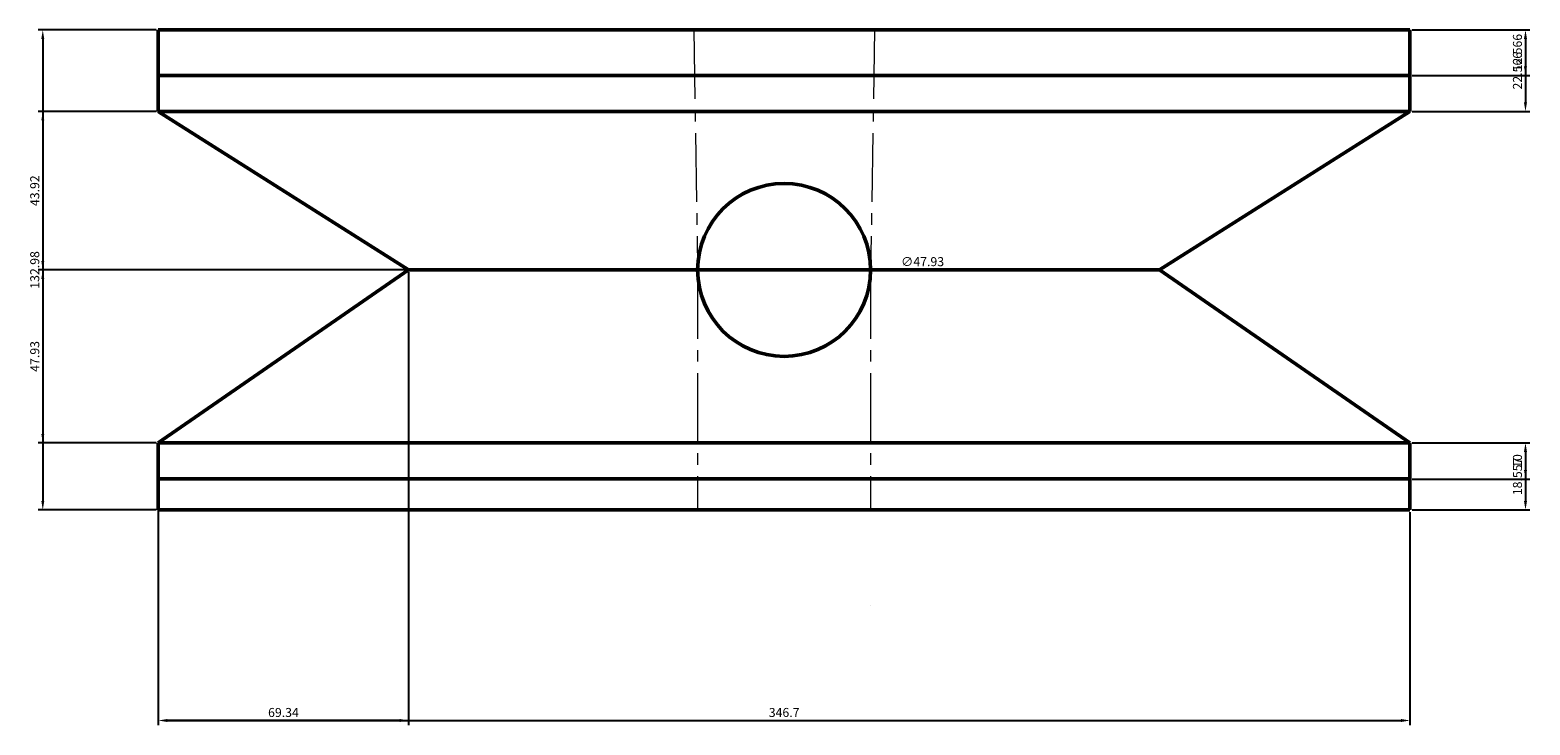
# Model space of a CAD drawing. Units: millimetres. Extents: x 921 to 2648, y 1390 to 2315.
# Tile 7 of 10: x 1771 to 2187, y 1657 to 1849. Entities that reach past the tile are written whole.
import ezdxf

# ---------------------------------------------------------------- set-up
doc = ezdxf.new("R2010")
doc.units = ezdxf.units.MM
doc.linetypes.add('CENTER2', pattern=[28.575, 19.05, -3.175, 3.175, -3.175])
for name, color, linetype, lineweight in [('M-CNTR', 1, 'CENTER2', 18), ('M-DIMS', 2, 'Continuous', 25), ('M-OUTL', 7, 'Continuous', 50)]:
    doc.layers.add(name, color=color, linetype=linetype, lineweight=lineweight)
doc.styles.get("Standard").update_dxf_attribs({"font": 'arial.ttf'})
doc.dimstyles.new('ISO-25', dxfattribs={"dimtxt": 2.5, "dimasz": 2.5, "dimexe": 1.25, "dimexo": 0.625, "dimtad": 1, "dimtxsty": 'Standard', "dimcen": 2.5, "dimadec": 0, "dimazin": 0, "dimtfac": 1, "dimtmove": 0, "dimatfit": 3, "dimfxl": 1, "dimarcsym": 0})

# ---------------------------------------------------------------- blocks, each defined once
blk = doc.blocks.new('*D34')
at = {"layer": 'Defpoints', "color": 0, "transparency": 16777216}
for p in [(1806.98, 1849.47), (1774.98, 1716.49), (1806.98, 1716.49)]:
    blk.add_point(p, dxfattribs=at)
at = {"layer": 'M-DIMS', "color": 0, "lineweight": -2, "transparency": 16777216}
for p, q in [((1806.36, 1849.47), (1773.73, 1849.47)), ((1774.98, 1846.97), (1774.98, 1718.99)), ((1806.36, 1716.49), (1773.73, 1716.49))]:
    blk.add_line(p, q, dxfattribs=at)
at = {"layer": 'M-DIMS', "color": 0, "transparency": 16777216}
for points in [[(1774.57, 1846.97), (1775.4, 1846.97), (1774.98, 1849.47)], [(1774.57, 1718.99), (1775.4, 1718.99), (1774.98, 1716.49)]]:
    blk.add_solid(points, dxfattribs=at)
at = {"layer": 'M-DIMS', "color": 0, "transparency": 16777216, "insert": (1773.08, 1782.98), "char_height": 2.5, "attachment_point": 5, "rotation": 90}
blk.add_mtext('132.98', dxfattribs=at)
blk = doc.blocks.new('*D83')
at = {"layer": 'Defpoints', "color": 0, "transparency": 16777216}
for p in [(1806.98, 1716.49), (2153.69, 1716.49), (2153.69, 1658.13)]:
    blk.add_point(p, dxfattribs=at)
at = {"layer": 'M-DIMS', "color": 0, "lineweight": -2, "transparency": 16777216}
for p, q in [((1806.98, 1715.87), (1806.98, 1656.88)), ((2153.69, 1715.87), (2153.69, 1656.88)), ((1809.48, 1658.13), (2151.19, 1658.13))]:
    blk.add_line(p, q, dxfattribs=at)
at = {"layer": 'M-DIMS', "color": 0, "transparency": 16777216}
for points in [[(1809.48, 1658.55), (1809.48, 1657.72), (1806.98, 1658.13)], [(2151.19, 1658.55), (2151.19, 1657.72), (2153.69, 1658.13)]]:
    blk.add_solid(points, dxfattribs=at)
at = {"layer": 'M-DIMS', "color": 0, "transparency": 16777216, "insert": (1980.34, 1660.03), "char_height": 2.5, "attachment_point": 5}
blk.add_mtext('346.7', dxfattribs=at)
blk = doc.blocks.new('*D84')
at = {"layer": 'Defpoints', "color": 0, "transparency": 16777216}
for p in [(2153.69, 1849.47), (2153.69, 1836.9), (2185.69, 1836.9)]:
    blk.add_point(p, dxfattribs=at)
at = {"layer": 'M-DIMS', "color": 0, "lineweight": -2, "transparency": 16777216}
for p, q in [((2154.32, 1849.47), (2186.94, 1849.47)), ((2185.69, 1846.97), (2185.69, 1839.4)), ((2154.32, 1836.9), (2186.94, 1836.9))]:
    blk.add_line(p, q, dxfattribs=at)
at = {"layer": 'M-DIMS', "color": 0, "transparency": 16777216}
for points in [[(2185.27, 1846.97), (2186.11, 1846.97), (2185.69, 1849.47)], [(2185.27, 1839.4), (2186.11, 1839.4), (2185.69, 1836.9)]]:
    blk.add_solid(points, dxfattribs=at)
at = {"layer": 'M-DIMS', "color": 0, "transparency": 16777216, "insert": (2183.79, 1843.19), "char_height": 2.5, "attachment_point": 5, "rotation": 90}
blk.add_mtext('12.566', dxfattribs=at)
blk = doc.blocks.new('*D85')
at = {"layer": 'Defpoints', "color": 0, "transparency": 16777216}
for p in [(2153.69, 1849.47), (2153.69, 1826.9), (2185.69, 1826.9)]:
    blk.add_point(p, dxfattribs=at)
at = {"layer": 'M-DIMS', "color": 0, "lineweight": -2, "transparency": 16777216}
for p, q in [((2154.32, 1849.47), (2186.94, 1849.47)), ((2185.69, 1846.97), (2185.69, 1829.4)), ((2154.32, 1826.9), (2186.94, 1826.9))]:
    blk.add_line(p, q, dxfattribs=at)
at = {"layer": 'M-DIMS', "color": 0, "transparency": 16777216}
for points in [[(2185.27, 1846.97), (2186.11, 1846.97), (2185.69, 1849.47)], [(2185.27, 1829.4), (2186.11, 1829.4), (2185.69, 1826.9)]]:
    blk.add_solid(points, dxfattribs=at)
at = {"layer": 'M-DIMS', "color": 0, "transparency": 16777216, "insert": (2183.79, 1838.19), "char_height": 2.5, "attachment_point": 5, "rotation": 90}
blk.add_mtext('22.566', dxfattribs=at)
blk = doc.blocks.new('*D86')
at = {"layer": 'Defpoints', "color": 0, "transparency": 16777216}
for p in [(2153.69, 1735.05), (2153.69, 1725.05), (2185.69, 1725.05)]:
    blk.add_point(p, dxfattribs=at)
at = {"layer": 'M-DIMS', "color": 0, "lineweight": -2, "transparency": 16777216}
for p, q in [((2154.32, 1735.05), (2186.94, 1735.05)), ((2185.69, 1732.55), (2185.69, 1727.55)), ((2154.32, 1725.05), (2186.94, 1725.05))]:
    blk.add_line(p, q, dxfattribs=at)
at = {"layer": 'M-DIMS', "color": 0, "transparency": 16777216}
for points in [[(2185.27, 1732.55), (2186.11, 1732.55), (2185.69, 1735.05)], [(2185.27, 1727.55), (2186.11, 1727.55), (2185.69, 1725.05)]]:
    blk.add_solid(points, dxfattribs=at)
at = {"layer": 'M-DIMS', "color": 0, "transparency": 16777216, "insert": (2183.79, 1730.05), "char_height": 2.5, "attachment_point": 5, "rotation": 90}
blk.add_mtext('10', dxfattribs=at)
blk = doc.blocks.new('*D87')
at = {"layer": 'Defpoints', "color": 0, "transparency": 16777216}
for p in [(2153.69, 1735.05), (2153.69, 1716.49), (2185.69, 1716.49)]:
    blk.add_point(p, dxfattribs=at)
at = {"layer": 'M-DIMS', "color": 0, "lineweight": -2, "transparency": 16777216}
for p, q in [((2154.32, 1735.05), (2186.94, 1735.05)), ((2185.69, 1732.55), (2185.69, 1718.99)), ((2154.32, 1716.49), (2186.94, 1716.49))]:
    blk.add_line(p, q, dxfattribs=at)
at = {"layer": 'M-DIMS', "color": 0, "transparency": 16777216}
for points in [[(2185.27, 1732.55), (2186.11, 1732.55), (2185.69, 1735.05)], [(2185.27, 1718.99), (2186.11, 1718.99), (2185.69, 1716.49)]]:
    blk.add_solid(points, dxfattribs=at)
at = {"layer": 'M-DIMS', "color": 0, "transparency": 16777216, "insert": (2183.79, 1725.77), "char_height": 2.5, "attachment_point": 5, "rotation": 90}
blk.add_mtext('18.557', dxfattribs=at)
blk = doc.blocks.new('*D88')
at = {"layer": 'Defpoints', "color": 0, "transparency": 16777216}
for p in [(1806.98, 1826.9), (1774.98, 1782.98), (1876.32, 1782.98)]:
    blk.add_point(p, dxfattribs=at)
at = {"layer": 'M-DIMS', "color": 0, "lineweight": -2, "transparency": 16777216}
for p, q in [((1806.36, 1826.9), (1773.73, 1826.9)), ((1774.98, 1824.4), (1774.98, 1785.48)), ((1875.7, 1782.98), (1773.73, 1782.98))]:
    blk.add_line(p, q, dxfattribs=at)
at = {"layer": 'M-DIMS', "color": 0, "transparency": 16777216}
for points in [[(1774.57, 1824.4), (1775.4, 1824.4), (1774.98, 1826.9)], [(1774.57, 1785.48), (1775.4, 1785.48), (1774.98, 1782.98)]]:
    blk.add_solid(points, dxfattribs=at)
at = {"layer": 'M-DIMS', "color": 0, "transparency": 16777216, "insert": (1773.08, 1804.94), "char_height": 2.5, "attachment_point": 5, "rotation": 90}
blk.add_mtext('43.92', dxfattribs=at)
blk = doc.blocks.new('*D89')
at = {"layer": 'Defpoints', "color": 0, "transparency": 16777216}
for p in [(1876.32, 1782.98), (1774.98, 1735.05), (1806.98, 1735.05)]:
    blk.add_point(p, dxfattribs=at)
at = {"layer": 'M-DIMS', "color": 0, "lineweight": -2, "transparency": 16777216}
for p, q in [((1875.7, 1782.98), (1773.73, 1782.98)), ((1774.98, 1780.48), (1774.98, 1737.55)), ((1806.36, 1735.05), (1773.73, 1735.05))]:
    blk.add_line(p, q, dxfattribs=at)
at = {"layer": 'M-DIMS', "color": 0, "transparency": 16777216}
for points in [[(1774.57, 1780.48), (1775.4, 1780.48), (1774.98, 1782.98)], [(1774.57, 1737.55), (1775.4, 1737.55), (1774.98, 1735.05)]]:
    blk.add_solid(points, dxfattribs=at)
at = {"layer": 'M-DIMS', "color": 0, "transparency": 16777216, "insert": (1773.08, 1759.02), "char_height": 2.5, "attachment_point": 5, "rotation": 90}
blk.add_mtext('47.93', dxfattribs=at)
blk = doc.blocks.new('*D90')
at = {"layer": 'Defpoints', "color": 0, "transparency": 16777216}
for p in [(1876.32, 1782.98), (1806.98, 1735.05), (1806.98, 1658.13)]:
    blk.add_point(p, dxfattribs=at)
at = {"layer": 'M-DIMS', "color": 0, "lineweight": -2, "transparency": 16777216}
for p, q in [((1876.32, 1782.36), (1876.32, 1656.88)), ((1806.98, 1734.43), (1806.98, 1656.88)), ((1873.82, 1658.13), (1809.48, 1658.13))]:
    blk.add_line(p, q, dxfattribs=at)
at = {"layer": 'M-DIMS', "color": 0, "transparency": 16777216}
for points in [[(1809.48, 1658.55), (1809.48, 1657.72), (1806.98, 1658.13)], [(1873.82, 1658.55), (1873.82, 1657.72), (1876.32, 1658.13)]]:
    blk.add_solid(points, dxfattribs=at)
at = {"layer": 'M-DIMS', "color": 0, "transparency": 16777216, "insert": (1841.65, 1660.03), "char_height": 2.5, "attachment_point": 5}
blk.add_mtext('69.34', dxfattribs=at)
blk = doc.blocks.new('*D118')
at = {"layer": 'Defpoints', "color": 0, "transparency": 16777216}
for p in [(1956.37, 1782.98), (2004.3, 1782.98)]:
    blk.add_point(p, dxfattribs=at)
at = {"layer": 'M-DIMS', "color": 0, "lineweight": -2, "transparency": 16777216}
for p, q in [((1953.87, 1782.98), (1951.37, 1782.98)), ((1956.37, 1782.98), (2004.3, 1782.98)), ((2024.89, 1782.98), (2006.8, 1782.98))]:
    blk.add_line(p, q, dxfattribs=at)
at = {"layer": 'M-DIMS', "color": 0, "transparency": 16777216}
for points in [[(1953.87, 1783.4), (1953.87, 1782.57), (1956.37, 1782.98)], [(2006.8, 1783.4), (2006.8, 1782.57), (2004.3, 1782.98)]]:
    blk.add_solid(points, dxfattribs=at)
at = {"layer": 'M-DIMS', "color": 0, "transparency": 16777216, "insert": (2018.68, 1784.95), "char_height": 2.5, "attachment_point": 5, "rotation": 0.0007}
blk.add_mtext('∅47.93', dxfattribs=at)

msp = doc.modelspace()

# ---------------------------------------------------------------- linework, layer by layer
at = {"layer": 'M-CNTR'}
for p, q in [((1955.2929, 1849.4706), (1956.3715, 1782.9827)), ((2005.3813, 1849.4706), (2004.3027, 1782.9827)), ((1956.3715, 1782.9827), (1956.3715, 1716.4948)), ((2004.3027, 1782.9827), (2004.3027, 1716.4948)), ((2004.3027, 1690.1325), (2004.3027, 1690.1325))]:
    msp.add_line(p, q, dxfattribs=at)
at = {"layer": 'M-OUTL'}
for p, q in [((1806.9834, 1849.4706), (2153.6909, 1849.4706)), ((1806.9834, 1849.4706), (1806.9834, 1826.9048)), ((2153.6909, 1849.4706), (2153.6909, 1826.9048)), ((1806.9834, 1836.9048), (2153.6909, 1836.9048)), ((2153.6909, 1826.9048), (1806.9834, 1826.9048)), ((1806.9834, 1826.9048), (1876.3249, 1782.9827)), ((2084.3494, 1782.9827), (2153.6909, 1826.9048)), ((1876.3249, 1782.9827), (1806.9834, 1735.0515)), ((1876.3249, 1782.9827), (2084.3494, 1782.9827)), ((2084.3494, 1782.9827), (2153.6909, 1735.0515)), ((2153.6909, 1735.0515), (1806.9834, 1735.0515)), ((1806.9834, 1735.0515), (1806.9834, 1716.4948)), ((2153.6909, 1735.0515), (2153.6909, 1716.4948)), ((1806.9834, 1725.0515), (2153.6909, 1725.0515)), ((2153.6909, 1716.4948), (1806.9834, 1716.4948))]:
    msp.add_line(p, q, dxfattribs=at)
msp.add_circle((1980.3371, 1782.9827), 23.9656, dxfattribs=at)

# ---------------------------------------------------------------- dimensions: what is measured, and where the dimension line sits
at = {"layer": 'M-DIMS'}
for base, p1, p2, override, picture, middle in [((1774.9834, 1716.4948), (1806.9834, 1849.4706), (1806.9834, 1716.4948), {"dimdec": 2, "dimlfac": 1, "dimrnd": 0, "dimzin": 0, "dimdsep": 46, "dimlunit": 2}, '*D34', (1773.0811, 1782.9827)), ((2185.6909, 1836.9048), (2153.6909, 1849.4706), (2153.6909, 1836.9048), {"dimdec": 3, "dimlfac": 1, "dimrnd": 0, "dimzin": 0, "dimdsep": 46, "dimlunit": 2}, '*D84', (2183.7894, 1843.1877)), ((2185.6909, 1826.9048), (2153.6909, 1849.4706), (2153.6909, 1826.9048), {"dimdec": 3, "dimlfac": 1, "dimrnd": 0, "dimzin": 0, "dimdsep": 46, "dimlunit": 2}, '*D85', (2183.7894, 1838.1877)), ((1774.9834, 1782.9827), (1806.9834, 1826.9048), (1876.3249, 1782.9827), {"dimdec": 2, "dimlfac": 1, "dimrnd": 0, "dimzin": 0, "dimdsep": 46, "dimlunit": 2}, '*D88', (1773.0811, 1804.9437)), ((1774.9834, 1735.0515), (1876.3249, 1782.9827), (1806.9834, 1735.0515), {"dimdec": 2, "dimlfac": 1, "dimrnd": 0, "dimzin": 0, "dimdsep": 46, "dimlunit": 2}, '*D89', (1773.0811, 1759.0171)), ((2185.6909, 1725.0515), (2153.6909, 1735.0515), (2153.6909, 1725.0515), {"dimdec": 0, "dimlfac": 1, "dimrnd": 0, "dimzin": 0, "dimdsep": 46, "dimlunit": 2}, '*D86', (2183.7894, 1730.0515)), ((2185.6909, 1716.4948), (2153.6909, 1735.0515), (2153.6909, 1716.4948), {"dimdec": 3, "dimlfac": 1, "dimrnd": 0, "dimzin": 0, "dimdsep": 46, "dimlunit": 2}, '*D87', (2183.7894, 1725.7732))]:
    dim = msp.add_linear_dim(base=base, p1=p1, p2=p2, angle=90, dimstyle='ISO-25', override=override, dxfattribs=at)
    dim.commit()
    dim.dimension.update_dxf_attribs({"geometry": picture, "text_midpoint": middle})
for base, p1, p2, override, picture, middle in [((1806.9834, 1658.1325), (1876.3249, 1782.9827), (1806.9834, 1735.0515), {"dimdec": 2, "dimlfac": 1, "dimrnd": 0, "dimzin": 0, "dimdsep": 46, "dimlunit": 2}, '*D90', (1841.6541, 1660.0348)), ((2153.6909, 1658.1325), (1806.9834, 1716.4948), (2153.6909, 1716.4948), {"dimdec": 1, "dimlfac": 1, "dimrnd": 0, "dimzin": 0, "dimdsep": 46, "dimlunit": 2}, '*D83', (1980.3371, 1660.0348))]:
    dim = msp.add_linear_dim(base=base, p1=p1, p2=p2, dimstyle='ISO-25', override=override, dxfattribs=at)
    dim.commit()
    dim.dimension.update_dxf_attribs({"geometry": picture, "text_midpoint": middle})
dim = msp.add_diameter_dim_2p(p1=(1956.3715, 1782.9824), p2=(2004.3027, 1782.983), dimstyle='ISO-25', override={"dimdec": 2, "dimlfac": 1, "dimrnd": 0, "dimzin": 0, "dimdsep": 46, "dimlunit": 2}, dxfattribs=at)
dim.commit()
dim.dimension.update_dxf_attribs({"geometry": '*D118', "text_midpoint": (2018.682, 1782.9832), "dimtype": 163})

doc.saveas('drawing.dxf')
